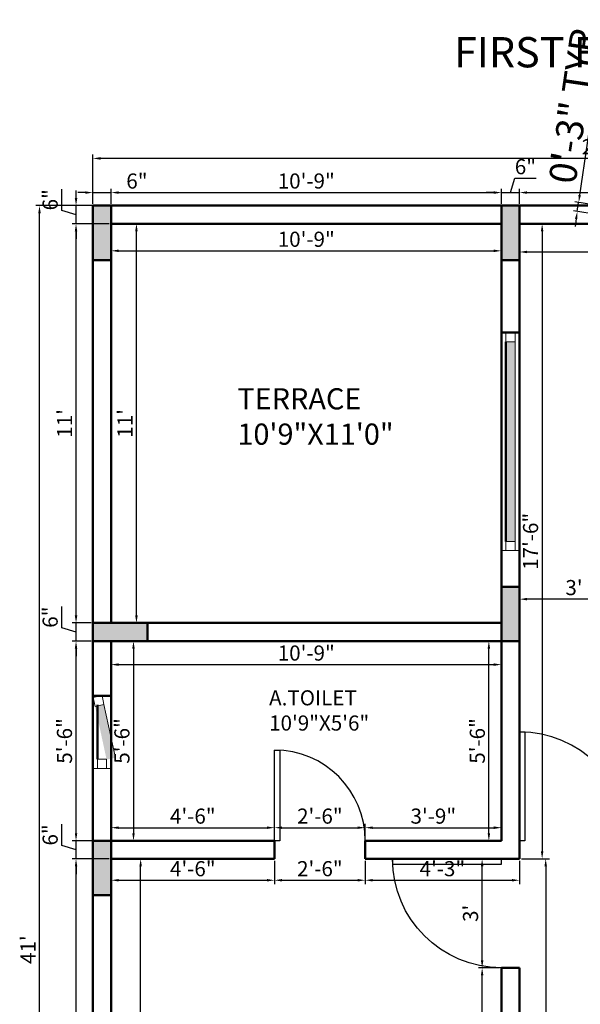
# Model space of a CAD drawing. Units: inches. Extents: x 3064 to 19385, y 846 to 15425.
# Tile 54 of 108: x 6445 to 6630, y 1132 to 1458. Entities that reach past the tile are written whole.
import ezdxf

# ---------------------------------------------------------------- set-up
doc = ezdxf.new("R2010")
doc.units = ezdxf.units.IN
for name, color, linetype, lineweight in [('A-ANNO-DIMS', 2, 'Continuous', 18), ('A-ANNO-TEXT', 7, 'Continuous', 25), ('A-AREA-IDEN', 3, 'Continuous', 18), ('A-COLS', 1, 'Continuous', 35), ('A-DOOR', 3, 'Continuous', 25), ('A-GLAZ', 4, 'Continuous', 18), ('A-WALL', 7, 'Continuous', 50)]:
    doc.layers.add(name, color=color, linetype=linetype, lineweight=lineweight)
doc.styles.get("Standard").update_dxf_attribs({"font": 'arial.ttf'})
doc.dimstyles.new('ISO-25', dxfattribs={"dimtxt": 9, "dimasz": 2.5, "dimexe": 1.25, "dimexo": 0.625, "dimtad": 1, "dimdec": 1, "dimlunit": 3, "dimtxsty": 'Standard', "dimcen": 2.5, "dimadec": 0, "dimazin": 0, "dimtfac": 1, "dimtdec": 1, "dimtmove": 0, "dimatfit": 3, "dimfxl": 1, "dimarcsym": 0})

# ---------------------------------------------------------------- blocks, each defined once
blk = doc.blocks.new('*U3')
for p, q in [((0, 0), (0, -6)), ((36, 0), (36, -6))]:
    blk.add_line(p, q)
blk.add_lwpolyline([(0, 0), (0, 36), (1.75, 36), (1.75, 0)], close=True)
blk.add_arc((0, 0), 36, 0, 90)
blk = doc.blocks.new('*U4')
for p, q in [((0, 0), (0, -6)), ((30, 0), (30, -6))]:
    blk.add_line(p, q)
blk.add_lwpolyline([(0, 0), (0, 30), (1.75, 30), (1.75, 0)], close=True)
blk.add_arc((0, 0), 30, 0, 90)
blk = doc.blocks.new('*D128')
at = {"layer": 'A-ANNO-DIMS', "color": 0, "lineweight": -2, "transparency": 16777216}
for p, q in [((6474.41, 1180.34), (6462.18, 1180.34)), ((6463.43, 984.84), (6463.43, 1177.84)), ((6474.41, 982.34), (6462.18, 982.34))]:
    blk.add_line(p, q, dxfattribs=at)
at = {"layer": 'A-ANNO-DIMS', "color": 0, "transparency": 16777216}
for points in [[(6463.02, 1177.84), (6463.85, 1177.84), (6463.43, 1180.34)], [(6463.02, 984.84), (6463.85, 984.84), (6463.43, 982.34)]]:
    blk.add_solid(points, dxfattribs=at)
at = {"layer": 'Defpoints', "color": 0, "transparency": 16777216}
for p in [(6463.43, 1180.34), (6475.03, 1180.34), (6475.03, 982.34)]:
    blk.add_point(p, dxfattribs=at)
at = {"layer": 'A-ANNO-DIMS', "color": 0, "transparency": 16777216, "insert": (6460.26, 1081.34), "char_height": 5, "attachment_point": 5, "rotation": 90}
blk.add_mtext('16\'-6"', dxfattribs=at)
blk = doc.blocks.new('*D129')
at = {"layer": 'A-ANNO-DIMS', "color": 0, "lineweight": -2, "transparency": 16777216}
for p, q in [((6458.69, 1184.76), (6458.69, 1191.79)), ((6463.43, 1188.84), (6463.43, 1191.34)), ((6474.41, 1186.34), (6462.18, 1186.34)), ((6463.43, 1180.34), (6463.43, 1186.34)), ((6463.43, 1180.34), (6463.43, 1186.34)), ((6463.43, 1183.34), (6458.69, 1184.76)), ((6474.41, 1180.34), (6462.18, 1180.34)), ((6463.43, 1177.84), (6463.43, 1175.34))]:
    blk.add_line(p, q, dxfattribs=at)
at = {"layer": 'A-ANNO-DIMS', "color": 0, "transparency": 16777216}
for points in [[(6463.02, 1188.84), (6463.85, 1188.84), (6463.43, 1186.34)], [(6463.02, 1177.84), (6463.85, 1177.84), (6463.43, 1180.34)]]:
    blk.add_solid(points, dxfattribs=at)
at = {"layer": 'Defpoints', "color": 0, "transparency": 16777216}
for p in [(6463.43, 1186.34), (6475.03, 1186.34), (6475.03, 1180.34)]:
    blk.add_point(p, dxfattribs=at)
at = {"layer": 'A-ANNO-DIMS', "color": 0, "transparency": 16777216, "insert": (6455.52, 1188.27), "char_height": 5, "attachment_point": 5, "rotation": 90}
blk.add_mtext('6"', dxfattribs=at)
blk = doc.blocks.new('*D130')
at = {"layer": 'A-ANNO-DIMS', "color": 0, "lineweight": -2, "transparency": 16777216}
for p, q in [((6468.41, 1252.34), (6462.18, 1252.34)), ((6463.43, 1188.84), (6463.43, 1249.84)), ((6474.41, 1186.34), (6462.18, 1186.34))]:
    blk.add_line(p, q, dxfattribs=at)
at = {"layer": 'A-ANNO-DIMS', "color": 0, "transparency": 16777216}
for points in [[(6463.02, 1249.84), (6463.85, 1249.84), (6463.43, 1252.34)], [(6463.02, 1188.84), (6463.85, 1188.84), (6463.43, 1186.34)]]:
    blk.add_solid(points, dxfattribs=at)
at = {"layer": 'Defpoints', "color": 0, "transparency": 16777216}
for p in [(6463.43, 1252.34), (6469.03, 1252.34), (6475.03, 1186.34)]:
    blk.add_point(p, dxfattribs=at)
at = {"layer": 'A-ANNO-DIMS', "color": 0, "transparency": 16777216, "insert": (6460.26, 1219.34), "char_height": 5, "attachment_point": 5, "rotation": 90}
blk.add_mtext('5\'-6"', dxfattribs=at)
blk = doc.blocks.new('*D123')
at = {"layer": 'A-ANNO-DIMS', "color": 0, "lineweight": -2, "transparency": 16777216}
for p, q in [((6458.69, 1256.76), (6458.69, 1263.79)), ((6463.43, 1260.84), (6463.43, 1263.34)), ((6463.43, 1255.34), (6458.69, 1256.76)), ((6468.41, 1258.34), (6462.18, 1258.34)), ((6463.43, 1252.34), (6463.43, 1258.34)), ((6463.43, 1252.34), (6463.43, 1258.34)), ((6468.41, 1252.34), (6462.18, 1252.34)), ((6463.43, 1249.84), (6463.43, 1247.34))]:
    blk.add_line(p, q, dxfattribs=at)
at = {"layer": 'A-ANNO-DIMS', "color": 0, "transparency": 16777216}
for points in [[(6463.02, 1260.84), (6463.85, 1260.84), (6463.43, 1258.34)], [(6463.02, 1249.84), (6463.85, 1249.84), (6463.43, 1252.34)]]:
    blk.add_solid(points, dxfattribs=at)
at = {"layer": 'Defpoints', "color": 0, "transparency": 16777216}
for p in [(6463.43, 1258.34), (6469.03, 1258.34), (6469.03, 1252.34)]:
    blk.add_point(p, dxfattribs=at)
at = {"layer": 'A-ANNO-DIMS', "color": 0, "transparency": 16777216, "insert": (6455.52, 1260.27), "char_height": 5, "attachment_point": 5, "rotation": 90}
blk.add_mtext('6"', dxfattribs=at)
blk = doc.blocks.new('*D124')
at = {"layer": 'A-ANNO-DIMS', "color": 0, "lineweight": -2, "transparency": 16777216}
for p, q in [((6474.41, 1390.34), (6462.18, 1390.34)), ((6463.43, 1260.84), (6463.43, 1387.84)), ((6468.41, 1258.34), (6462.18, 1258.34))]:
    blk.add_line(p, q, dxfattribs=at)
at = {"layer": 'A-ANNO-DIMS', "color": 0, "transparency": 16777216}
for points in [[(6463.02, 1387.84), (6463.85, 1387.84), (6463.43, 1390.34)], [(6463.02, 1260.84), (6463.85, 1260.84), (6463.43, 1258.34)]]:
    blk.add_solid(points, dxfattribs=at)
at = {"layer": 'Defpoints', "color": 0, "transparency": 16777216}
for p in [(6463.43, 1390.34), (6475.03, 1390.34), (6469.03, 1258.34)]:
    blk.add_point(p, dxfattribs=at)
at = {"layer": 'A-ANNO-DIMS', "color": 0, "transparency": 16777216, "insert": (6460.3, 1324.34), "char_height": 5, "attachment_point": 5, "rotation": 90}
blk.add_mtext("11'", dxfattribs=at)
blk = doc.blocks.new('*D125')
at = {"layer": 'A-ANNO-DIMS', "color": 0, "lineweight": -2, "transparency": 16777216}
for p, q in [((6458.69, 1394.76), (6458.69, 1401.79)), ((6463.43, 1398.84), (6463.43, 1401.34)), ((6463.43, 1393.34), (6458.69, 1394.76)), ((6474.41, 1396.34), (6462.18, 1396.34)), ((6463.43, 1390.34), (6463.43, 1396.34)), ((6463.43, 1390.34), (6463.43, 1396.34)), ((6474.41, 1390.34), (6462.18, 1390.34)), ((6463.43, 1387.84), (6463.43, 1385.34))]:
    blk.add_line(p, q, dxfattribs=at)
at = {"layer": 'A-ANNO-DIMS', "color": 0, "transparency": 16777216}
for points in [[(6463.02, 1398.84), (6463.85, 1398.84), (6463.43, 1396.34)], [(6463.02, 1387.84), (6463.85, 1387.84), (6463.43, 1390.34)]]:
    blk.add_solid(points, dxfattribs=at)
at = {"layer": 'Defpoints', "color": 0, "transparency": 16777216}
for p in [(6463.43, 1396.34), (6475.03, 1396.34), (6475.03, 1390.34)]:
    blk.add_point(p, dxfattribs=at)
at = {"layer": 'A-ANNO-DIMS', "color": 0, "transparency": 16777216, "insert": (6455.52, 1398.27), "char_height": 5, "attachment_point": 5, "rotation": 90}
blk.add_mtext('6"', dxfattribs=at)
blk = doc.blocks.new('*D126')
at = {"layer": 'A-ANNO-DIMS', "color": 0, "lineweight": -2, "transparency": 16777216}
for p, q in [((6468.41, 1396.34), (6450.1, 1396.34)), ((6451.35, 906.84), (6451.35, 1393.84)), ((6468.41, 904.34), (6450.1, 904.34))]:
    blk.add_line(p, q, dxfattribs=at)
at = {"layer": 'A-ANNO-DIMS', "color": 0, "transparency": 16777216}
for points in [[(6450.94, 1393.84), (6451.77, 1393.84), (6451.35, 1396.34)], [(6450.94, 906.84), (6451.77, 906.84), (6451.35, 904.34)]]:
    blk.add_solid(points, dxfattribs=at)
at = {"layer": 'Defpoints', "color": 0, "transparency": 16777216}
for p in [(6451.35, 1396.34), (6469.03, 1396.34), (6469.03, 904.34)]:
    blk.add_point(p, dxfattribs=at)
at = {"layer": 'A-ANNO-DIMS', "color": 0, "transparency": 16777216, "insert": (6448.22, 1150.34), "char_height": 5, "attachment_point": 5, "rotation": 90}
blk.add_mtext("41'", dxfattribs=at)
blk = doc.blocks.new('*D97')
at = {"layer": 'A-ANNO-DIMS', "color": 0, "lineweight": -2, "transparency": 16777216}
for p, q in [((6466.53, 1400.65), (6464.03, 1400.65)), ((6469.03, 1396.96), (6469.03, 1401.9)), ((6469.03, 1400.65), (6475.03, 1400.65)), ((6475.03, 1396.96), (6475.03, 1401.9)), ((6477.53, 1400.65), (6487.06, 1400.65))]:
    blk.add_line(p, q, dxfattribs=at)
at = {"layer": 'A-ANNO-DIMS', "color": 0, "transparency": 16777216}
for points in [[(6466.53, 1401.07), (6466.53, 1400.24), (6469.03, 1400.65)], [(6477.53, 1401.07), (6477.53, 1400.24), (6475.03, 1400.65)]]:
    blk.add_solid(points, dxfattribs=at)
at = {"layer": 'Defpoints', "color": 0, "transparency": 16777216}
for p in [(6475.03, 1400.65), (6469.03, 1396.34), (6475.03, 1396.34)]:
    blk.add_point(p, dxfattribs=at)
at = {"layer": 'A-ANNO-DIMS', "color": 0, "transparency": 16777216, "insert": (6483.55, 1403.83), "char_height": 5, "attachment_point": 5}
blk.add_mtext('6"', dxfattribs=at)
blk = doc.blocks.new('*D105')
at = {"layer": 'A-ANNO-DIMS', "color": 0, "lineweight": -2, "transparency": 16777216}
for p, q in [((6475.03, 1396.96), (6475.03, 1401.9)), ((6477.53, 1400.65), (6601.53, 1400.65)), ((6604.03, 1396.96), (6604.03, 1401.9))]:
    blk.add_line(p, q, dxfattribs=at)
at = {"layer": 'A-ANNO-DIMS', "color": 0, "transparency": 16777216}
for points in [[(6477.53, 1401.07), (6477.53, 1400.24), (6475.03, 1400.65)], [(6601.53, 1401.07), (6601.53, 1400.24), (6604.03, 1400.65)]]:
    blk.add_solid(points, dxfattribs=at)
at = {"layer": 'Defpoints', "color": 0, "transparency": 16777216}
for p in [(6604.03, 1400.65), (6475.03, 1396.34), (6604.03, 1396.34)]:
    blk.add_point(p, dxfattribs=at)
at = {"layer": 'A-ANNO-DIMS', "color": 0, "transparency": 16777216, "insert": (6539.53, 1403.83), "char_height": 5, "attachment_point": 5}
blk.add_mtext('10\'-9"', dxfattribs=at)
blk = doc.blocks.new('*D99')
at = {"layer": 'A-ANNO-DIMS', "color": 0, "lineweight": -2, "transparency": 16777216}
for p, q in [((6607.03, 1400.65), (6608.46, 1405.39)), ((6608.46, 1405.39), (6615.48, 1405.39)), ((6601.53, 1400.65), (6599.03, 1400.65)), ((6604.03, 1396.96), (6604.03, 1401.9)), ((6604.03, 1400.65), (6610.03, 1400.65)), ((6604.03, 1400.65), (6610.03, 1400.65)), ((6610.03, 1396.96), (6610.03, 1401.9)), ((6612.53, 1400.65), (6615.03, 1400.65))]:
    blk.add_line(p, q, dxfattribs=at)
at = {"layer": 'A-ANNO-DIMS', "color": 0, "transparency": 16777216}
for points in [[(6601.53, 1401.07), (6601.53, 1400.24), (6604.03, 1400.65)], [(6612.53, 1401.07), (6612.53, 1400.24), (6610.03, 1400.65)]]:
    blk.add_solid(points, dxfattribs=at)
at = {"layer": 'Defpoints', "color": 0, "transparency": 16777216}
for p in [(6610.03, 1400.65), (6604.03, 1396.34), (6610.03, 1396.34)]:
    blk.add_point(p, dxfattribs=at)
at = {"layer": 'A-ANNO-DIMS', "color": 0, "transparency": 16777216, "insert": (6611.97, 1408.57), "char_height": 5, "attachment_point": 5}
blk.add_mtext('6"', dxfattribs=at)
blk = doc.blocks.new('*D100')
at = {"layer": 'A-ANNO-DIMS', "color": 0, "lineweight": -2, "transparency": 16777216}
for p, q in [((6610.03, 1396.96), (6610.03, 1401.9)), ((6612.53, 1400.65), (6802.53, 1400.65)), ((6805.03, 1396.96), (6805.03, 1401.9))]:
    blk.add_line(p, q, dxfattribs=at)
at = {"layer": 'A-ANNO-DIMS', "color": 0, "transparency": 16777216}
for points in [[(6612.53, 1401.07), (6612.53, 1400.24), (6610.03, 1400.65)], [(6802.53, 1401.07), (6802.53, 1400.24), (6805.03, 1400.65)]]:
    blk.add_solid(points, dxfattribs=at)
at = {"layer": 'Defpoints', "color": 0, "transparency": 16777216}
for p in [(6805.03, 1400.65), (6610.03, 1396.34), (6805.03, 1396.34)]:
    blk.add_point(p, dxfattribs=at)
at = {"layer": 'A-ANNO-DIMS', "color": 0, "transparency": 16777216, "insert": (6707.53, 1403.83), "char_height": 5, "attachment_point": 5}
blk.add_mtext('16\'-3"', dxfattribs=at)
blk = doc.blocks.new('*D96')
at = {"layer": 'A-ANNO-DIMS', "color": 0, "lineweight": -2, "transparency": 16777216}
for p, q in [((6469.03, 1396.96), (6469.03, 1413.2)), ((6811.03, 1396.96), (6811.03, 1413.2)), ((6808.53, 1411.95), (6471.53, 1411.95))]:
    blk.add_line(p, q, dxfattribs=at)
at = {"layer": 'A-ANNO-DIMS', "color": 0, "transparency": 16777216}
for points in [[(6471.53, 1412.37), (6471.53, 1411.53), (6469.03, 1411.95)], [(6808.53, 1412.37), (6808.53, 1411.53), (6811.03, 1411.95)]]:
    blk.add_solid(points, dxfattribs=at)
at = {"layer": 'Defpoints', "color": 0, "transparency": 16777216}
for p in [(6469.03, 1411.95), (6469.03, 1396.34), (6811.03, 1396.34)]:
    blk.add_point(p, dxfattribs=at)
at = {"layer": 'A-ANNO-DIMS', "color": 0, "transparency": 16777216, "insert": (6640.03, 1415.13), "char_height": 5, "attachment_point": 5}
blk.add_mtext('28\'-6"', dxfattribs=at)
blk = doc.blocks.new('*D188')
at = {"layer": 'A-ANNO-DIMS', "color": 0, "lineweight": -2, "transparency": 16777216}
for p, q in [((6475.66, 1180.34), (6486.03, 1180.34)), ((6484.78, 984.84), (6484.78, 1177.84)), ((6475.66, 982.34), (6486.03, 982.34))]:
    blk.add_line(p, q, dxfattribs=at)
at = {"layer": 'A-ANNO-DIMS', "color": 0, "transparency": 16777216}
for points in [[(6484.37, 1177.84), (6485.2, 1177.84), (6484.78, 1180.34)], [(6484.37, 984.84), (6485.2, 984.84), (6484.78, 982.34)]]:
    blk.add_solid(points, dxfattribs=at)
at = {"layer": 'Defpoints', "color": 0, "transparency": 16777216}
for p in [(6475.03, 1180.34), (6484.78, 1180.34), (6475.03, 982.34)]:
    blk.add_point(p, dxfattribs=at)
at = {"layer": 'A-ANNO-DIMS', "color": 0, "transparency": 16777216, "insert": (6481.6, 1081.34), "char_height": 5, "attachment_point": 5, "rotation": 90}
blk.add_mtext('16\'-6"', dxfattribs=at)
blk = doc.blocks.new('*D189')
at = {"layer": 'A-ANNO-DIMS', "color": 0, "lineweight": -2, "transparency": 16777216}
for p, q in [((6475.03, 1179.71), (6475.03, 1172.03)), ((6529.03, 1179.71), (6529.03, 1172.03)), ((6477.53, 1173.28), (6526.53, 1173.28))]:
    blk.add_line(p, q, dxfattribs=at)
at = {"layer": 'A-ANNO-DIMS', "color": 0, "transparency": 16777216}
for points in [[(6477.53, 1173.7), (6477.53, 1172.87), (6475.03, 1173.28)], [(6526.53, 1173.7), (6526.53, 1172.87), (6529.03, 1173.28)]]:
    blk.add_solid(points, dxfattribs=at)
at = {"layer": 'Defpoints', "color": 0, "transparency": 16777216}
for p in [(6475.03, 1180.34), (6529.03, 1180.34), (6529.03, 1173.28)]:
    blk.add_point(p, dxfattribs=at)
at = {"layer": 'A-ANNO-DIMS', "color": 0, "transparency": 16777216, "insert": (6502.03, 1176.46), "char_height": 5, "attachment_point": 5}
blk.add_mtext('4\'-6"', dxfattribs=at)
blk = doc.blocks.new('*D190')
at = {"layer": 'A-ANNO-DIMS', "color": 0, "lineweight": -2, "transparency": 16777216}
for p, q in [((6529.03, 1179.71), (6529.03, 1172.03)), ((6559.03, 1179.71), (6559.03, 1172.03)), ((6531.53, 1173.28), (6556.53, 1173.28))]:
    blk.add_line(p, q, dxfattribs=at)
at = {"layer": 'A-ANNO-DIMS', "color": 0, "transparency": 16777216}
for points in [[(6531.53, 1173.7), (6531.53, 1172.87), (6529.03, 1173.28)], [(6556.53, 1173.7), (6556.53, 1172.87), (6559.03, 1173.28)]]:
    blk.add_solid(points, dxfattribs=at)
at = {"layer": 'Defpoints', "color": 0, "transparency": 16777216}
for p in [(6529.03, 1180.34), (6559.03, 1180.34), (6559.03, 1173.28)]:
    blk.add_point(p, dxfattribs=at)
at = {"layer": 'A-ANNO-DIMS', "color": 0, "transparency": 16777216, "insert": (6544.03, 1176.46), "char_height": 5, "attachment_point": 5}
blk.add_mtext('2\'-6"', dxfattribs=at)
blk = doc.blocks.new('*D191')
at = {"layer": 'A-ANNO-DIMS', "color": 0, "lineweight": -2, "transparency": 16777216}
for p, q in [((6559.03, 1179.71), (6559.03, 1172.03)), ((6610.03, 1179.71), (6610.03, 1172.03)), ((6561.53, 1173.28), (6607.53, 1173.28))]:
    blk.add_line(p, q, dxfattribs=at)
at = {"layer": 'A-ANNO-DIMS', "color": 0, "transparency": 16777216}
for points in [[(6561.53, 1173.7), (6561.53, 1172.87), (6559.03, 1173.28)], [(6607.53, 1173.7), (6607.53, 1172.87), (6610.03, 1173.28)]]:
    blk.add_solid(points, dxfattribs=at)
at = {"layer": 'Defpoints', "color": 0, "transparency": 16777216}
for p in [(6559.03, 1180.34), (6610.03, 1180.34), (6610.03, 1173.28)]:
    blk.add_point(p, dxfattribs=at)
at = {"layer": 'A-ANNO-DIMS', "color": 0, "transparency": 16777216, "insert": (6584.53, 1176.46), "char_height": 5, "attachment_point": 5}
blk.add_mtext('4\'-3"', dxfattribs=at)
blk = doc.blocks.new('*D192')
at = {"layer": 'A-ANNO-DIMS', "color": 0, "lineweight": -2, "transparency": 16777216}
for p, q in [((6603.41, 1144.34), (6596.41, 1144.34)), ((6597.66, 984.84), (6597.66, 1141.84)), ((6603.41, 982.34), (6596.41, 982.34))]:
    blk.add_line(p, q, dxfattribs=at)
at = {"layer": 'A-ANNO-DIMS', "color": 0, "transparency": 16777216}
for points in [[(6597.25, 1141.84), (6598.08, 1141.84), (6597.66, 1144.34)], [(6597.25, 984.84), (6598.08, 984.84), (6597.66, 982.34)]]:
    blk.add_solid(points, dxfattribs=at)
at = {"layer": 'Defpoints', "color": 0, "transparency": 16777216}
for p in [(6597.66, 1144.34), (6604.03, 1144.34), (6604.03, 982.34)]:
    blk.add_point(p, dxfattribs=at)
at = {"layer": 'A-ANNO-DIMS', "color": 0, "transparency": 16777216, "insert": (6594.48, 1063.34), "char_height": 5, "attachment_point": 5, "rotation": 90}
blk.add_mtext('13\'-6"', dxfattribs=at)
blk = doc.blocks.new('*D193')
at = {"layer": 'A-ANNO-DIMS', "color": 0, "lineweight": -2, "transparency": 16777216}
for p, q in [((6598.29, 1180.34), (6598.91, 1180.34)), ((6597.66, 1146.84), (6597.66, 1177.84)), ((6603.41, 1144.34), (6596.41, 1144.34))]:
    blk.add_line(p, q, dxfattribs=at)
at = {"layer": 'A-ANNO-DIMS', "color": 0, "transparency": 16777216}
for points in [[(6597.25, 1177.84), (6598.08, 1177.84), (6597.66, 1180.34)], [(6597.25, 1146.84), (6598.08, 1146.84), (6597.66, 1144.34)]]:
    blk.add_solid(points, dxfattribs=at)
at = {"layer": 'Defpoints', "color": 0, "transparency": 16777216}
for p in [(6597.66, 1180.34), (6597.66, 1180.34), (6604.03, 1144.34)]:
    blk.add_point(p, dxfattribs=at)
at = {"layer": 'A-ANNO-DIMS', "color": 0, "transparency": 16777216, "insert": (6594.48, 1162.34), "char_height": 5, "attachment_point": 5, "rotation": 90}
blk.add_mtext("3'", dxfattribs=at)
blk = doc.blocks.new('*D194')
at = {"layer": 'A-ANNO-DIMS', "color": 0, "lineweight": -2, "transparency": 16777216}
for p, q in [((6475.03, 1186.96), (6475.03, 1191.91)), ((6529.03, 1186.96), (6529.03, 1191.91)), ((6477.53, 1190.66), (6526.53, 1190.66))]:
    blk.add_line(p, q, dxfattribs=at)
at = {"layer": 'A-ANNO-DIMS', "color": 0, "transparency": 16777216}
for points in [[(6477.53, 1191.08), (6477.53, 1190.24), (6475.03, 1190.66)], [(6526.53, 1191.08), (6526.53, 1190.24), (6529.03, 1190.66)]]:
    blk.add_solid(points, dxfattribs=at)
at = {"layer": 'Defpoints', "color": 0, "transparency": 16777216}
for p in [(6529.03, 1190.66), (6475.03, 1186.34), (6529.03, 1186.34)]:
    blk.add_point(p, dxfattribs=at)
at = {"layer": 'A-ANNO-DIMS', "color": 0, "transparency": 16777216, "insert": (6502.03, 1193.84), "char_height": 5, "attachment_point": 5}
blk.add_mtext('4\'-6"', dxfattribs=at)
blk = doc.blocks.new('*D195')
at = {"layer": 'A-ANNO-DIMS', "color": 0, "lineweight": -2, "transparency": 16777216}
for p, q in [((6529.03, 1186.96), (6529.03, 1191.91)), ((6559.03, 1186.96), (6559.03, 1191.91)), ((6531.53, 1190.66), (6556.53, 1190.66))]:
    blk.add_line(p, q, dxfattribs=at)
at = {"layer": 'A-ANNO-DIMS', "color": 0, "transparency": 16777216}
for points in [[(6531.53, 1191.08), (6531.53, 1190.24), (6529.03, 1190.66)], [(6556.53, 1191.08), (6556.53, 1190.24), (6559.03, 1190.66)]]:
    blk.add_solid(points, dxfattribs=at)
at = {"layer": 'Defpoints', "color": 0, "transparency": 16777216}
for p in [(6559.03, 1190.66), (6529.03, 1186.34), (6559.03, 1186.34)]:
    blk.add_point(p, dxfattribs=at)
at = {"layer": 'A-ANNO-DIMS', "color": 0, "transparency": 16777216, "insert": (6544.03, 1193.84), "char_height": 5, "attachment_point": 5}
blk.add_mtext('2\'-6"', dxfattribs=at)
blk = doc.blocks.new('*D196')
at = {"layer": 'A-ANNO-DIMS', "color": 0, "lineweight": -2, "transparency": 16777216}
for p, q in [((6559.03, 1186.96), (6559.03, 1191.91)), ((6604.03, 1186.96), (6604.03, 1191.91)), ((6561.53, 1190.66), (6601.53, 1190.66))]:
    blk.add_line(p, q, dxfattribs=at)
at = {"layer": 'A-ANNO-DIMS', "color": 0, "transparency": 16777216}
for points in [[(6561.53, 1191.08), (6561.53, 1190.24), (6559.03, 1190.66)], [(6601.53, 1191.08), (6601.53, 1190.24), (6604.03, 1190.66)]]:
    blk.add_solid(points, dxfattribs=at)
at = {"layer": 'Defpoints', "color": 0, "transparency": 16777216}
for p in [(6604.03, 1190.66), (6559.03, 1186.34), (6604.03, 1186.34)]:
    blk.add_point(p, dxfattribs=at)
at = {"layer": 'A-ANNO-DIMS', "color": 0, "transparency": 16777216, "insert": (6581.53, 1193.84), "char_height": 5, "attachment_point": 5}
blk.add_mtext('3\'-9"', dxfattribs=at)
blk = doc.blocks.new('*D197')
at = {"layer": 'A-ANNO-DIMS', "color": 0, "lineweight": -2, "transparency": 16777216}
for p, q in [((6603.41, 1252.34), (6598.64, 1252.34)), ((6599.89, 1188.84), (6599.89, 1249.84)), ((6603.41, 1186.34), (6598.64, 1186.34))]:
    blk.add_line(p, q, dxfattribs=at)
at = {"layer": 'A-ANNO-DIMS', "color": 0, "transparency": 16777216}
for points in [[(6599.48, 1249.84), (6600.31, 1249.84), (6599.89, 1252.34)], [(6599.48, 1188.84), (6600.31, 1188.84), (6599.89, 1186.34)]]:
    blk.add_solid(points, dxfattribs=at)
at = {"layer": 'Defpoints', "color": 0, "transparency": 16777216}
for p in [(6599.89, 1252.34), (6604.03, 1252.34), (6604.03, 1186.34)]:
    blk.add_point(p, dxfattribs=at)
at = {"layer": 'A-ANNO-DIMS', "color": 0, "transparency": 16777216, "insert": (6596.72, 1219.34), "char_height": 5, "attachment_point": 5, "rotation": 90}
blk.add_mtext('5\'-6"', dxfattribs=at)
blk = doc.blocks.new('*D198')
at = {"layer": 'A-ANNO-DIMS', "color": 0, "lineweight": -2, "transparency": 16777216}
for p, q in [((6475.03, 1251.71), (6475.03, 1243.33)), ((6604.03, 1251.71), (6604.03, 1243.33)), ((6477.53, 1244.58), (6601.53, 1244.58))]:
    blk.add_line(p, q, dxfattribs=at)
at = {"layer": 'A-ANNO-DIMS', "color": 0, "transparency": 16777216}
for points in [[(6477.53, 1245), (6477.53, 1244.16), (6475.03, 1244.58)], [(6601.53, 1245), (6601.53, 1244.16), (6604.03, 1244.58)]]:
    blk.add_solid(points, dxfattribs=at)
at = {"layer": 'Defpoints', "color": 0, "transparency": 16777216}
for p in [(6475.03, 1252.34), (6604.03, 1252.34), (6604.03, 1244.58)]:
    blk.add_point(p, dxfattribs=at)
at = {"layer": 'A-ANNO-DIMS', "color": 0, "transparency": 16777216, "insert": (6539.53, 1247.76), "char_height": 5, "attachment_point": 5}
blk.add_mtext('10\'-9"', dxfattribs=at)
blk = doc.blocks.new('*D199')
at = {"layer": 'A-ANNO-DIMS', "color": 0, "lineweight": -2, "transparency": 16777216}
for p, q in [((6475.66, 1252.34), (6483.67, 1252.34)), ((6482.42, 1249.84), (6482.42, 1188.84)), ((6475.66, 1186.34), (6483.67, 1186.34))]:
    blk.add_line(p, q, dxfattribs=at)
at = {"layer": 'A-ANNO-DIMS', "color": 0, "transparency": 16777216}
for points in [[(6482.01, 1249.84), (6482.84, 1249.84), (6482.42, 1252.34)], [(6482.01, 1188.84), (6482.84, 1188.84), (6482.42, 1186.34)]]:
    blk.add_solid(points, dxfattribs=at)
at = {"layer": 'Defpoints', "color": 0, "transparency": 16777216}
for p in [(6475.03, 1252.34), (6475.03, 1186.34), (6482.42, 1186.34)]:
    blk.add_point(p, dxfattribs=at)
at = {"layer": 'A-ANNO-DIMS', "color": 0, "transparency": 16777216, "insert": (6479.25, 1219.34), "char_height": 5, "attachment_point": 5, "rotation": 90}
blk.add_mtext('5\'-6"', dxfattribs=at)
blk = doc.blocks.new('*D200')
at = {"layer": 'A-ANNO-DIMS', "color": 0, "lineweight": -2, "transparency": 16777216}
for p, q in [((6475.66, 1390.34), (6484.65, 1390.34)), ((6483.4, 1260.84), (6483.4, 1387.84)), ((6475.66, 1258.34), (6484.65, 1258.34))]:
    blk.add_line(p, q, dxfattribs=at)
at = {"layer": 'A-ANNO-DIMS', "color": 0, "transparency": 16777216}
for points in [[(6482.98, 1387.84), (6483.81, 1387.84), (6483.4, 1390.34)], [(6482.98, 1260.84), (6483.81, 1260.84), (6483.4, 1258.34)]]:
    blk.add_solid(points, dxfattribs=at)
at = {"layer": 'Defpoints', "color": 0, "transparency": 16777216}
for p in [(6475.03, 1390.34), (6483.4, 1390.34), (6475.03, 1258.34)]:
    blk.add_point(p, dxfattribs=at)
at = {"layer": 'A-ANNO-DIMS', "color": 0, "transparency": 16777216, "insert": (6480.26, 1324.34), "char_height": 5, "attachment_point": 5, "rotation": 90}
blk.add_mtext("11'", dxfattribs=at)
blk = doc.blocks.new('*D201')
at = {"layer": 'A-ANNO-DIMS', "color": 0, "lineweight": -2, "transparency": 16777216}
for p, q in [((6475.03, 1389.71), (6475.03, 1380.15)), ((6604.03, 1389.71), (6604.03, 1380.15)), ((6477.53, 1381.4), (6601.53, 1381.4))]:
    blk.add_line(p, q, dxfattribs=at)
at = {"layer": 'A-ANNO-DIMS', "color": 0, "transparency": 16777216}
for points in [[(6477.53, 1381.81), (6477.53, 1380.98), (6475.03, 1381.4)], [(6601.53, 1381.81), (6601.53, 1380.98), (6604.03, 1381.4)]]:
    blk.add_solid(points, dxfattribs=at)
at = {"layer": 'Defpoints', "color": 0, "transparency": 16777216}
for p in [(6475.03, 1390.34), (6604.03, 1390.34), (6604.03, 1381.4)]:
    blk.add_point(p, dxfattribs=at)
at = {"layer": 'A-ANNO-DIMS', "color": 0, "transparency": 16777216, "insert": (6539.53, 1384.57), "char_height": 5, "attachment_point": 5}
blk.add_mtext('10\'-9"', dxfattribs=at)
blk = doc.blocks.new('*D202')
at = {"layer": 'A-ANNO-DIMS', "color": 0, "lineweight": -2, "transparency": 16777216}
for p, q in [((6610.66, 1390.34), (6618.75, 1390.34)), ((6617.5, 1387.84), (6617.5, 1182.84)), ((6610.66, 1180.34), (6618.75, 1180.34))]:
    blk.add_line(p, q, dxfattribs=at)
at = {"layer": 'A-ANNO-DIMS', "color": 0, "transparency": 16777216}
for points in [[(6617.08, 1387.84), (6617.91, 1387.84), (6617.5, 1390.34)], [(6617.08, 1182.84), (6617.91, 1182.84), (6617.5, 1180.34)]]:
    blk.add_solid(points, dxfattribs=at)
at = {"layer": 'Defpoints', "color": 0, "transparency": 16777216}
for p in [(6610.03, 1390.34), (6610.03, 1180.34), (6617.5, 1180.34)]:
    blk.add_point(p, dxfattribs=at)
at = {"layer": 'A-ANNO-DIMS', "color": 0, "transparency": 16777216, "insert": (6614.32, 1285.34), "char_height": 5, "attachment_point": 5, "rotation": 90}
blk.add_mtext('17\'-6"', dxfattribs=at)
blk = doc.blocks.new('*D212')
at = {"layer": 'A-ANNO-DIMS', "color": 0, "lineweight": -2, "transparency": 16777216}
for p, q in [((6610.03, 1389.71), (6610.03, 1379.77)), ((6805.03, 1389.71), (6805.03, 1379.77)), ((6612.53, 1381.02), (6802.53, 1381.02))]:
    blk.add_line(p, q, dxfattribs=at)
at = {"layer": 'A-ANNO-DIMS', "color": 0, "transparency": 16777216}
for points in [[(6612.53, 1381.44), (6612.53, 1380.6), (6610.03, 1381.02)], [(6802.53, 1381.44), (6802.53, 1380.6), (6805.03, 1381.02)]]:
    blk.add_solid(points, dxfattribs=at)
at = {"layer": 'Defpoints', "color": 0, "transparency": 16777216}
for p in [(6610.03, 1390.34), (6805.03, 1390.34), (6805.03, 1381.02)]:
    blk.add_point(p, dxfattribs=at)
at = {"layer": 'A-ANNO-DIMS', "color": 0, "transparency": 16777216, "insert": (6707.53, 1384.2), "char_height": 5, "attachment_point": 5}
blk.add_mtext('16\'-3"', dxfattribs=at)
blk = doc.blocks.new('*D215')
at = {"layer": 'A-ANNO-DIMS', "color": 0, "lineweight": -2, "transparency": 16777216}
for p, q in [((6610.03, 1269.71), (6610.03, 1264.97)), ((6646.03, 1258.96), (6646.03, 1267.47)), ((6643.53, 1266.22), (6612.53, 1266.22))]:
    blk.add_line(p, q, dxfattribs=at)
at = {"layer": 'A-ANNO-DIMS', "color": 0, "transparency": 16777216}
for points in [[(6612.53, 1266.64), (6612.53, 1265.81), (6610.03, 1266.22)], [(6643.53, 1266.64), (6643.53, 1265.81), (6646.03, 1266.22)]]:
    blk.add_solid(points, dxfattribs=at)
at = {"layer": 'Defpoints', "color": 0, "transparency": 16777216}
for p in [(6610.03, 1270.34), (6610.03, 1266.22), (6646.03, 1258.34)]:
    blk.add_point(p, dxfattribs=at)
at = {"layer": 'A-ANNO-DIMS', "color": 0, "transparency": 16777216, "insert": (6628.03, 1269.4), "char_height": 5, "attachment_point": 5}
blk.add_mtext("3'", dxfattribs=at)
blk = doc.blocks.new('*D216')
at = {"layer": 'A-ANNO-DIMS', "color": 0, "lineweight": -2, "transparency": 16777216}
for p, q in [((6610.66, 1180.34), (6619.92, 1180.34)), ((6618.67, 1177.84), (6618.67, 984.84)), ((6610.66, 982.34), (6619.92, 982.34))]:
    blk.add_line(p, q, dxfattribs=at)
at = {"layer": 'A-ANNO-DIMS', "color": 0, "transparency": 16777216}
for points in [[(6618.26, 1177.84), (6619.09, 1177.84), (6618.67, 1180.34)], [(6618.26, 984.84), (6619.09, 984.84), (6618.67, 982.34)]]:
    blk.add_solid(points, dxfattribs=at)
at = {"layer": 'Defpoints', "color": 0, "transparency": 16777216}
for p in [(6610.03, 1180.34), (6610.03, 982.34), (6618.67, 982.34)]:
    blk.add_point(p, dxfattribs=at)
at = {"layer": 'A-ANNO-DIMS', "color": 0, "transparency": 16777216, "insert": (6615.5, 1081.34), "char_height": 5, "attachment_point": 5, "rotation": 90}
blk.add_mtext('16\'-6"', dxfattribs=at)
blk = doc.blocks.new('WIN-600')
h = blk.add_hatch(color=256)
h.dxf.hatch_style = 1
h.paths.add_polyline_path([(3, 18), (0, 18), (0, 0), (3, 0)])
blk.add_line((3, 18), (3, 0))
blk.add_lwpolyline([(3, 18), (0, 18), (0, 21), (3, 21)], close=True)
blk = doc.blocks.new('WIN-1900')
blk.add_line((3, 0), (3, 66))
blk.add_lwpolyline([(3, 66), (0, 66), (0, 69), (3, 69)], close=True)
blk = doc.blocks.new('*D438')
at = {"layer": 'A-ANNO-DIMS', "color": 0, "lineweight": -2, "transparency": 16777216}
for p, q in [((6629.92, 1399.83), (6638.45, 1457.82)), ((6633.84, 1396.73), (6628.32, 1397.54)), ((6629.12, 1394.39), (6629.56, 1397.36)), ((6633.4, 1393.76), (6627.89, 1394.57)), ((6628.76, 1391.92), (6628.4, 1389.44))]:
    blk.add_line(p, q, dxfattribs=at)
at = {"layer": 'A-ANNO-DIMS', "color": 0, "transparency": 16777216}
for points in [[(6629.51, 1399.89), (6630.34, 1399.77), (6629.56, 1397.36)], [(6628.35, 1391.98), (6629.17, 1391.86), (6629.12, 1394.39)]]:
    blk.add_solid(points, dxfattribs=at)
at = {"layer": 'Defpoints', "color": 0, "transparency": 16777216}
for p in [(6629.56, 1397.36), (6634.46, 1396.64), (6634.02, 1393.67)]:
    blk.add_point(p, dxfattribs=at)
at = {"layer": 'A-ANNO-DIMS', "color": 0, "transparency": 16777216, "insert": (6629.2, 1430.82), "char_height": 9, "attachment_point": 5, "rotation": 81.6351}
blk.add_mtext('0\'-3" TYP.', dxfattribs=at)

msp = doc.modelspace()

# ---------------------------------------------------------------- hatches: boundary and pattern name
at = {"layer": 'A-COLS'}
h = msp.add_hatch(color=256, dxfattribs=at)
h.dxf.hatch_style = 1
h.paths.add_polyline_path([(6469.03, 1378.34), (6475.03, 1378.34), (6475.03, 1396.34), (6469.03, 1396.34)])
h = msp.add_hatch(color=256, dxfattribs=at)
h.dxf.hatch_style = 1
h.paths.add_polyline_path([(6604.03, 1378.34), (6610.03, 1378.34), (6610.03, 1396.34), (6604.03, 1396.34)])
h = msp.add_hatch(color=256, dxfattribs=at)
h.dxf.hatch_style = 1
h.paths.add_polyline_path([(6604.03, 1252.34), (6610.03, 1252.34), (6610.03, 1270.34), (6604.03, 1270.34)])
h = msp.add_hatch(color=256, dxfattribs=at)
h.dxf.hatch_style = 1
h.paths.add_polyline_path([(6487.03, 1252.34), (6487.03, 1258.34), (6469.03, 1258.34), (6469.03, 1252.34)])
h = msp.add_hatch(color=256, dxfattribs=at)
h.dxf.hatch_style = 1
h.paths.add_polyline_path([(6469.03, 1168.34), (6475.03, 1168.34), (6475.03, 1186.34), (6469.03, 1186.34)])
at = {"layer": 'A-GLAZ'}
h = msp.add_hatch(color=256, dxfattribs=at)
h.dxf.hatch_style = 1
h.paths.add_polyline_path([(6605.53, 1285.34), (6608.53, 1285.34), (6608.53, 1351.34), (6605.53, 1351.34)])

# ---------------------------------------------------------------- linework, layer by layer
for p, q in [((6610.03, 1282.34), (6604.03, 1282.34)), ((6469.03, 1210.28), (6475.03, 1210.28))]:
    msp.add_line(p, q, dxfattribs=at)
for points in [[(6608.53, 1282.34), (6605.53, 1282.34), (6605.53, 1285.34), (6608.53, 1285.34)], [(6473.53, 1210.28), (6470.53, 1210.28), (6470.53, 1213.28), (6473.53, 1213.28)]]:
    msp.add_lwpolyline(points, close=True, dxfattribs=at)
at = {"layer": 'A-WALL'}
for p, q in [((6811.03, 1396.34), (6469.03, 1396.34)), ((6469.03, 1396.34), (6469.03, 976.34)), ((6604.03, 1390.34), (6475.03, 1390.34)), ((6475.03, 1390.34), (6475.03, 1258.34)), ((6604.03, 1390.34), (6604.03, 1258.34)), ((6805.03, 1390.34), (6610.03, 1390.34)), ((6610.03, 1390.34), (6610.03, 1180.34)), ((6604.03, 1354.34), (6610.03, 1354.34)), ((6605.53, 1351.34), (6605.53, 1285.34)), ((6475.03, 1258.34), (6604.03, 1258.34)), ((6475.03, 1252.34), (6475.03, 1186.34)), ((6475.03, 1252.34), (6604.03, 1252.34)), ((6610.03, 1252.34), (6604.03, 1252.34)), ((6604.03, 1252.34), (6604.03, 1186.34)), ((6469.03, 1234.28), (6475.03, 1234.28)), ((6470.53, 1231.28), (6470.53, 1213.28)), ((6475.03, 1186.34), (6529.03, 1186.34)), ((6529.03, 1186.34), (6529.03, 1180.34)), ((6559.03, 1186.34), (6604.03, 1186.34)), ((6559.03, 1186.34), (6559.03, 1180.34)), ((6475.03, 1180.34), (6475.03, 982.34)), ((6475.03, 1180.34), (6529.03, 1180.34)), ((6559.03, 1180.34), (6610.03, 1180.34)), ((6604.03, 1144.34), (6604.03, 982.34)), ((6604.03, 1144.34), (6610.03, 1144.34)), ((6610.03, 1144.34), (6610.03, 976.34))]:
    msp.add_line(p, q, dxfattribs=at)
for points in [[(6475.03, 1378.34), (6475.03, 1396.34), (6469.03, 1396.34), (6469.03, 1378.34)], [(6610.03, 1378.34), (6610.03, 1396.34), (6604.03, 1396.34), (6604.03, 1378.34)], [(6610.03, 1252.34), (6610.03, 1270.34), (6604.03, 1270.34), (6604.03, 1252.34)], [(6487.03, 1258.34), (6469.03, 1258.34), (6469.03, 1252.34), (6487.03, 1252.34)], [(6475.03, 1168.34), (6475.03, 1186.34), (6469.03, 1186.34), (6469.03, 1168.34)]]:
    msp.add_lwpolyline(points, close=True, dxfattribs=at)

# ---------------------------------------------------------------- block references
at = {"layer": 'A-DOOR'}
for name, p in [('*U3', (6610.03, 1186.34)), ('*U4', (6529.03, 1186.34))]:
    msp.add_blockref(name, p, dxfattribs=at)
at = {"layer": 'A-DOOR', "xscale": -1, "rotation": 90}
msp.add_blockref('*U3', (6604.03, 1180.34), dxfattribs=at)
at = {"layer": 'A-GLAZ'}
msp.add_blockref('WIN-1900', (6605.53, 1285.34), dxfattribs=at)
at = {"layer": 'A-GLAZ', "rotation": 12.21571913413091}
msp.add_blockref('WIN-600', (6473.54, 1213.17), dxfattribs=at)

# ---------------------------------------------------------------- texts
at = {"layer": 'A-ANNO-TEXT', "insert": (6588.38, 1452.06), "char_height": 10, "attachment_point": 1}
msp.add_mtext_dynamic_manual_height_columns('FIRST FLOOR PLAN', width=200.9739, gutter_width=12.5, heights=[0], dxfattribs=at)
at = {"layer": 'A-AREA-IDEN', "attachment_point": 1}
for s, insert, char_height in [('TERRACE\\P10\'9"X11\'0"', (6516.76, 1335.96), 7), ('A.TOILET\\P10\'9"X5\'6"', (6527.25, 1236.1), 5)]:
    msp.add_mtext_dynamic_manual_height_columns(s, width=67.5924, gutter_width=12.5, heights=[0], dxfattribs=dict(at, insert=insert, char_height=char_height))

# ---------------------------------------------------------------- dimensions: what is measured, and where the dimension line sits
at = {"layer": 'A-ANNO-DIMS'}
dim = msp.add_linear_dim(base=(6629.56, 1397.36), p1=(6634.02, 1393.67), p2=(6634.46, 1396.64), angle=81.6351, text='<> TYP.', dimstyle='ISO-25', override={"dimdec": 1, "dimrnd": 0, "dimzin": 1, "dimlunit": 4, "dimfrac": 2}, dxfattribs=at)
dim.commit()
dim.dimension.update_dxf_attribs({"geometry": '*D438', "text_midpoint": (6629.2, 1430.82)})
for base, p1, p2, override, picture, middle in [((6469.03, 1411.95), (6811.03, 1396.34), (6469.03, 1396.34), {"dimtxt": 5, "dimclrd": 0, "dimclre": 0, "dimclrt": 0}, '*D96', (6640.03, 1415.13)), ((6610.03, 1400.65), (6604.03, 1396.34), (6610.03, 1396.34), {"dimtxt": 5, "dimclrd": 0, "dimclre": 0, "dimclrt": 0, "dimtmove": 1}, '*D99', (6609.08, 1408.57)), ((6475.03, 1400.65), (6469.03, 1396.34), (6475.03, 1396.34), {"dimtxt": 5, "dimclrd": 0, "dimclre": 0, "dimclrt": 0}, '*D97', (6483.55, 1403.83)), ((6604.03, 1400.65), (6475.03, 1396.34), (6604.03, 1396.34), {"dimtxt": 5, "dimclrd": 0, "dimclre": 0, "dimclrt": 0, "dimtmove": 1}, '*D105', (6539.53, 1403.83)), ((6805.03, 1400.65), (6610.03, 1396.34), (6805.03, 1396.34), {"dimtxt": 5, "dimclrd": 0, "dimclre": 0, "dimclrt": 0, "dimtmove": 1}, '*D100', (6707.53, 1403.83)), ((6604.03, 1381.4), (6475.03, 1390.34), (6604.03, 1390.34), {"dimtxt": 5, "dimclrd": 0, "dimclre": 0, "dimclrt": 0}, '*D201', (6539.53, 1384.57)), ((6805.03, 1381.02), (6610.03, 1390.34), (6805.03, 1390.34), {"dimtxt": 5, "dimclrd": 0, "dimclre": 0, "dimclrt": 0}, '*D212', (6707.53, 1384.2)), ((6610.03, 1266.22), (6646.03, 1258.34), (6610.03, 1270.34), {"dimtxt": 5, "dimclrd": 0, "dimclre": 0, "dimclrt": 0, "dimtmove": 1}, '*D215', (6628.03, 1269.4)), ((6604.03, 1244.58), (6475.03, 1252.34), (6604.03, 1252.34), {"dimtxt": 5, "dimclrd": 0, "dimclre": 0, "dimclrt": 0}, '*D198', (6539.53, 1247.76)), ((6529.03, 1190.66), (6475.03, 1186.34), (6529.03, 1186.34), {"dimtxt": 5, "dimclrd": 0, "dimclre": 0, "dimclrt": 0}, '*D194', (6502.03, 1193.84)), ((6559.03, 1190.66), (6529.03, 1186.34), (6559.03, 1186.34), {"dimtxt": 5, "dimclrd": 0, "dimclre": 0, "dimclrt": 0, "dimtmove": 1}, '*D195', (6544.03, 1193.84)), ((6604.03, 1190.66), (6559.03, 1186.34), (6604.03, 1186.34), {"dimtxt": 5, "dimclrd": 0, "dimclre": 0, "dimclrt": 0, "dimtmove": 1}, '*D196', (6581.53, 1193.84)), ((6529.03, 1173.28), (6475.03, 1180.34), (6529.03, 1180.34), {"dimtxt": 5, "dimclrd": 0, "dimclre": 0, "dimclrt": 0}, '*D189', (6502.03, 1176.46)), ((6559.03, 1173.28), (6529.03, 1180.34), (6559.03, 1180.34), {"dimtxt": 5, "dimclrd": 0, "dimclre": 0, "dimclrt": 0, "dimtmove": 1}, '*D190', (6544.03, 1176.46)), ((6610.03, 1173.28), (6559.03, 1180.34), (6610.03, 1180.34), {"dimtxt": 5, "dimclrd": 0, "dimclre": 0, "dimclrt": 0, "dimtmove": 1}, '*D191', (6584.53, 1176.46))]:
    dim = msp.add_linear_dim(base=base, p1=p1, p2=p2, dimstyle='ISO-25', override=override, dxfattribs=at)
    dim.commit()
    dim.dimension.update_dxf_attribs({"geometry": picture, "text_midpoint": middle})
for base, p1, p2, override, picture, middle in [((6463.43, 1396.34), (6475.03, 1390.34), (6475.03, 1396.34), {"dimtxt": 5, "dimclrd": 0, "dimclre": 0, "dimclrt": 0, "dimtmove": 1}, '*D125', (6455.52, 1395.39)), ((6451.35, 1396.34), (6469.03, 904.34), (6469.03, 1396.34), {"dimtxt": 5, "dimclrd": 0, "dimclre": 0, "dimclrt": 0}, '*D126', (6448.22, 1150.34)), ((6463.43, 1390.34), (6469.03, 1258.34), (6475.03, 1390.34), {"dimtxt": 5, "dimclrd": 0, "dimclre": 0, "dimclrt": 0, "dimtmove": 1}, '*D124', (6460.3, 1324.34)), ((6483.4, 1390.34), (6475.03, 1258.34), (6475.03, 1390.34), {"dimtxt": 5, "dimclrd": 0, "dimclre": 0, "dimclrt": 0}, '*D200', (6480.26, 1324.34)), ((6617.5, 1180.34), (6610.03, 1390.34), (6610.03, 1180.34), {"dimtxt": 5, "dimclrd": 0, "dimclre": 0, "dimclrt": 0}, '*D202', (6614.32, 1285.34)), ((6463.43, 1258.34), (6469.03, 1252.34), (6469.03, 1258.34), {"dimtxt": 5, "dimclrd": 0, "dimclre": 0, "dimclrt": 0, "dimtmove": 1}, '*D123', (6455.52, 1257.39)), ((6463.43, 1252.34), (6475.03, 1186.34), (6469.03, 1252.34), {"dimtxt": 5, "dimclrd": 0, "dimclre": 0, "dimclrt": 0, "dimtmove": 1}, '*D130', (6460.26, 1219.34)), ((6482.42, 1186.34), (6475.03, 1252.34), (6475.03, 1186.34), {"dimtxt": 5, "dimclrd": 0, "dimclre": 0, "dimclrt": 0}, '*D199', (6479.25, 1219.34)), ((6599.89, 1252.34), (6604.03, 1186.34), (6604.03, 1252.34), {"dimtxt": 5, "dimclrd": 0, "dimclre": 0, "dimclrt": 0}, '*D197', (6596.72, 1219.34)), ((6463.43, 1186.34), (6475.03, 1180.34), (6475.03, 1186.34), {"dimtxt": 5, "dimclrd": 0, "dimclre": 0, "dimclrt": 0, "dimtmove": 1}, '*D129', (6455.52, 1185.39)), ((6463.43, 1180.34), (6475.03, 982.34), (6475.03, 1180.34), {"dimtxt": 5, "dimclrd": 0, "dimclre": 0, "dimclrt": 0, "dimtmove": 1}, '*D128', (6460.26, 1081.34)), ((6484.78, 1180.34), (6475.03, 982.34), (6475.03, 1180.34), {"dimtxt": 5, "dimclrd": 0, "dimclre": 0, "dimclrt": 0}, '*D188', (6481.6, 1081.34)), ((6597.66, 1180.34), (6604.03, 1144.34), (6597.66, 1180.34), {"dimtxt": 5, "dimclrd": 0, "dimclre": 0, "dimclrt": 0, "dimtmove": 1}, '*D193', (6594.48, 1162.34)), ((6618.67, 982.34), (6610.03, 1180.34), (6610.03, 982.34), {"dimtxt": 5, "dimclrd": 0, "dimclre": 0, "dimclrt": 0}, '*D216', (6615.5, 1081.34)), ((6597.66, 1144.34), (6604.03, 982.34), (6604.03, 1144.34), {"dimtxt": 5, "dimclrd": 0, "dimclre": 0, "dimclrt": 0}, '*D192', (6594.48, 1063.34))]:
    dim = msp.add_linear_dim(base=base, p1=p1, p2=p2, angle=90, dimstyle='ISO-25', override=override, dxfattribs=at)
    dim.commit()
    dim.dimension.update_dxf_attribs({"geometry": picture, "text_midpoint": middle})

doc.saveas('drawing.dxf')
